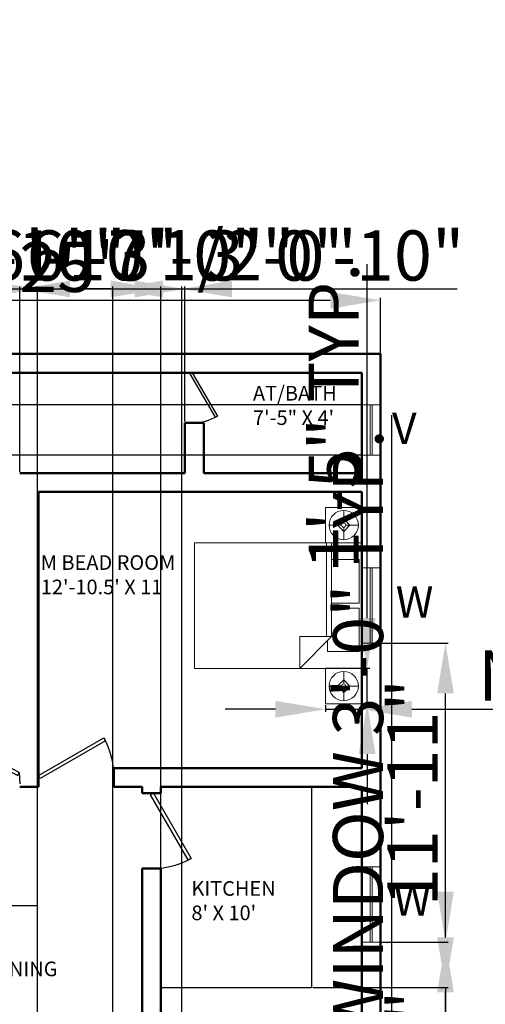
# Model space of a CAD drawing. Units: inches. Extents: x 1383 to 2465, y 1661 to 2415.
# Tile 3 of 4: x 1880 to 2102, y 1944 to 2415. Entities that reach past the tile are written whole.
import ezdxf

# ---------------------------------------------------------------- set-up
doc = ezdxf.new("R2010")
doc.units = ezdxf.units.IN
for name, color, linetype, lineweight in [('A-ANNO-DIMS', 2, 'Continuous', 18), ('A-ANNO-TEXT', 3, 'Continuous', 18), ('A-AREA-IDEN', 7, 'Continuous', 25), ('A-DOOR', 3, 'Continuous', 25), ('A-FLOR-FIXT', 9, 'Continuous', 25), ('A-FURN', 8, 'Continuous', 18), ('A-GLAZ', 4, 'Continuous', 18), ('A-WALL', 7, 'Continuous', 50)]:
    doc.layers.add(name, color=color, linetype=linetype, lineweight=lineweight)
doc.styles.get("Standard").update_dxf_attribs({"font": 'arial.ttf'})
doc.dimstyles.new('ISO-25', dxfattribs={"dimtxt": 24, "dimasz": 24, "dimexe": 1.25, "dimexo": 0.625, "dimtad": 1, "dimdec": 0, "dimlunit": 3, "dimtxsty": 'Standard', "dimcen": 2.5, "dimadec": 0, "dimazin": 0, "dimtfac": 1, "dimtdec": 0, "dimtmove": 0, "dimatfit": 3, "dimfxl": 1, "dimarcsym": 0})

# ---------------------------------------------------------------- blocks, each defined once
blk = doc.blocks.new('*U2')
for p, q in [((0, 0), (0, -6)), ((40, 0), (40, -6))]:
    blk.add_line(p, q)
blk.add_lwpolyline([(0, 0), (34.64, 20), (35.52, 18.48), (0.87, -1.52)], close=True)
blk.add_arc((0, 0), 40, 0, 30)
blk = doc.blocks.new('*U4')
for p, q in [((0, 0), (0, -6)), ((-40, 0), (-40, -6))]:
    blk.add_line(p, q)
blk.add_lwpolyline([(0, 0), (-34.64, 20), (-35.52, 18.48), (-0.88, -1.52)], close=True)
blk.add_arc((0, 0), 40, 150, 180)
blk = doc.blocks.new('*U5')
for p, q in [((-40, 0), (-40, 6)), ((0, 0), (0, 6))]:
    blk.add_line(p, q)
blk.add_lwpolyline([(0, 0), (-34.64, -20), (-35.52, -18.48), (-0.88, 1.52)], close=True)
blk.add_arc((0, 0), 40, 180, 210)
blk = doc.blocks.new('Bed - Queen')
for p, q in [((0, -80.00003), (0, 0)), ((0, 0), (59.99999, 0)), ((59.99999, 0), (59.99999, -80.00003)), ((7.99999, -1.2), (28.79998, -1.2)), ((7.99999, -14.4), (7.99999, -1.2)), ((28.79998, -1.2), (28.79998, -14.4)), ((31.19999, -1.2), (51.99999, -1.2)), ((31.19999, -14.4), (31.19999, -1.2)), ((51.99999, -1.2), (51.99999, -16.4)), ((0, -14.4), (44.8, -14.4)), ((44.8, -16.8), (0, -16.8)), ((59.99999, -29.6), (44.8, -14.4)), ((44.8, -14.4), (44.8, -29.6)), ((51.99999, -16.4), (46.79936, -16.4)), ((44.8, -29.6), (59.99999, -29.6)), ((59.99999, -80.00003), (0, -80.00003))]:
    blk.add_line(p, q)
blk = doc.blocks.new('*D12')
at = {"layer": 'A-ANNO-DIMS', "color": 0, "lineweight": -2, "transparency": 16777216}
for p, q in [((1752.19, 2255.79), (1752.19, 2282.04)), ((1776.19, 2280.79), (2028.19, 2280.79)), ((2052.19, 2255.79), (2052.19, 2282.04))]:
    blk.add_line(p, q, dxfattribs=at)
at = {"layer": 'A-ANNO-DIMS', "color": 0, "transparency": 16777216}
for points in [[(1776.19, 2284.79), (1776.19, 2276.79), (1752.19, 2280.79)], [(2028.19, 2284.79), (2028.19, 2276.79), (2052.19, 2280.79)]]:
    blk.add_solid(points, dxfattribs=at)
at = {"layer": 'Defpoints', "color": 0, "transparency": 16777216}
for p in [(2052.19, 2280.79), (1752.19, 2255.16), (2052.19, 2255.16)]:
    blk.add_point(p, dxfattribs=at)
at = {"layer": 'A-ANNO-DIMS', "color": 0, "transparency": 16777216, "insert": (1902.19, 2293.67), "char_height": 24, "attachment_point": 5}
blk.add_mtext("25'", dxfattribs=at)
blk = doc.blocks.new('WIN-36IN')
for p, q in [((0, 36), (9, 36)), ((0, 0), (0, 36)), ((4, 0), (4, 36)), ((5, 36), (5, 0)), ((9, 36), (9, 0)), ((9, 0), (0, 0))]:
    blk.add_line(p, q)
blk = doc.blocks.new('Lamp - Table')
for p, q in [((0, 7), (0, 1)), ((-1, 0), (-7, 0)), ((0, 3), (-3, 0)), ((-3, 0), (0, -3)), ((3, 0), (0, 3)), ((0, -3), (3, 0)), ((1, 0), (7, 0)), ((0, -1), (0, -7))]:
    blk.add_line(p, q)
for radius in [7, 1]:
    blk.add_circle((0, 0), radius)
blk = doc.blocks.new('NIGHTSTAND-WITH-LAMP')
blk.add_lwpolyline([(0, 0), (17.23, 0), (17.23, 16.98), (0, 16.98)], close=True)
blk.add_blockref('Lamp - Table', (8.62, 8.49))
blk = doc.blocks.new('*D16')
at = {"layer": 'A-ANNO-DIMS', "color": 0, "lineweight": -2, "transparency": 16777216}
for p, q in [((2025.96, 2087.24), (2025.96, 2084.03)), ((2043.19, 2087.24), (2043.19, 2084.03)), ((2001.96, 2085.28), (1977.96, 2085.28)), ((2025.96, 2085.28), (2043.19, 2085.28)), ((2067.19, 2085.28), (2464.82, 2085.28))]:
    blk.add_line(p, q, dxfattribs=at)
at = {"layer": 'A-ANNO-DIMS', "color": 0, "transparency": 16777216}
for points in [[(2001.96, 2089.28), (2001.96, 2081.28), (2025.96, 2085.28)], [(2067.19, 2089.28), (2067.19, 2081.28), (2043.19, 2085.28)]]:
    blk.add_solid(points, dxfattribs=at)
at = {"layer": 'Defpoints', "color": 0, "transparency": 16777216}
for p in [(2025.96, 2087.86), (2043.19, 2087.86), (2043.19, 2085.28)]:
    blk.add_point(p, dxfattribs=at)
at = {"layer": 'A-ANNO-DIMS', "color": 0, "transparency": 16777216, "insert": (2278.01, 2098.31), "char_height": 24, "attachment_point": 5}
blk.add_mtext('NIGHTSTAND 1\'-5" TYP.', dxfattribs=at)
blk = doc.blocks.new('*D17')
at = {"layer": 'A-ANNO-DIMS', "color": 0, "lineweight": -2, "transparency": 16777216}
for p, q in [((2045.78, 2128.84), (2045.78, 2298.12)), ((2043.82, 2104.84), (2047.03, 2104.84)), ((2045.78, 2087.86), (2045.78, 2104.84)), ((2043.82, 2087.86), (2047.03, 2087.86)), ((2045.78, 2063.86), (2045.78, 2039.86))]:
    blk.add_line(p, q, dxfattribs=at)
at = {"layer": 'A-ANNO-DIMS', "color": 0, "transparency": 16777216}
for points in [[(2041.78, 2128.84), (2049.78, 2128.84), (2045.78, 2104.84)], [(2041.78, 2063.86), (2049.78, 2063.86), (2045.78, 2087.86)]]:
    blk.add_solid(points, dxfattribs=at)
at = {"layer": 'Defpoints', "color": 0, "transparency": 16777216}
for p in [(2043.19, 2104.84), (2045.78, 2104.84), (2043.19, 2087.86)]:
    blk.add_point(p, dxfattribs=at)
at = {"layer": 'A-ANNO-DIMS', "color": 0, "transparency": 16777216, "insert": (2032.9, 2225.48), "char_height": 24, "attachment_point": 5, "rotation": 90}
blk.add_mtext('1\'-5" TYP.', dxfattribs=at)
blk = doc.blocks.new('*D18')
at = {"layer": 'A-ANNO-DIMS', "color": 0, "lineweight": -2, "transparency": 16777216}
for p, q in [((2057.59, 1896.91), (2057.59, 2225.86)), ((2052.82, 1872.91), (2058.84, 1872.91)), ((2057.59, 1836.91), (2057.59, 1872.91)), ((2052.82, 1836.91), (2058.84, 1836.91)), ((2057.59, 1812.91), (2057.59, 1788.91))]:
    blk.add_line(p, q, dxfattribs=at)
at = {"layer": 'A-ANNO-DIMS', "color": 0, "transparency": 16777216}
for points in [[(2053.59, 1896.91), (2061.59, 1896.91), (2057.59, 1872.91)], [(2053.59, 1812.91), (2061.59, 1812.91), (2057.59, 1836.91)]]:
    blk.add_solid(points, dxfattribs=at)
at = {"layer": 'Defpoints', "color": 0, "transparency": 16777216}
for p in [(2052.19, 1872.91), (2057.59, 1872.91), (2052.19, 1836.91)]:
    blk.add_point(p, dxfattribs=at)
at = {"layer": 'A-ANNO-DIMS', "color": 0, "transparency": 16777216, "insert": (2044.54, 2073.39), "char_height": 24, "attachment_point": 5, "rotation": 90}
blk.add_mtext('WINDOW 3\'-0" TYP.', dxfattribs=at)
blk = doc.blocks.new('*D32')
at = {"layer": 'A-ANNO-DIMS', "color": 0, "lineweight": -2, "transparency": 16777216}
for p, q in [((2052.82, 1973.98), (2084.49, 1973.98)), ((2083.24, 1860.91), (2083.24, 1949.98)), ((2052.82, 1836.91), (2084.49, 1836.91))]:
    blk.add_line(p, q, dxfattribs=at)
at = {"layer": 'A-ANNO-DIMS', "color": 0, "transparency": 16777216}
for points in [[(2079.24, 1949.98), (2087.24, 1949.98), (2083.24, 1973.98)], [(2079.24, 1860.91), (2087.24, 1860.91), (2083.24, 1836.91)]]:
    blk.add_solid(points, dxfattribs=at)
at = {"layer": 'Defpoints', "color": 0, "transparency": 16777216}
for p in [(2052.19, 1973.98), (2083.24, 1973.98), (2052.19, 1836.91)]:
    blk.add_point(p, dxfattribs=at)
at = {"layer": 'A-ANNO-DIMS', "color": 0, "transparency": 16777216, "insert": (2070.36, 1905.44), "char_height": 24, "attachment_point": 5, "rotation": 90}
blk.add_mtext('11\'-5"', dxfattribs=at)
blk = doc.blocks.new('*D33')
at = {"layer": 'A-ANNO-DIMS', "color": 0, "lineweight": -2, "transparency": 16777216}
for p, q in [((2052.82, 2116.87), (2084.49, 2116.87)), ((2083.24, 1997.98), (2083.24, 2092.87)), ((2052.82, 1973.98), (2084.49, 1973.98))]:
    blk.add_line(p, q, dxfattribs=at)
at = {"layer": 'A-ANNO-DIMS', "color": 0, "transparency": 16777216}
for points in [[(2079.24, 2092.87), (2087.24, 2092.87), (2083.24, 2116.87)], [(2079.24, 1997.98), (2087.24, 1997.98), (2083.24, 1973.98)]]:
    blk.add_solid(points, dxfattribs=at)
at = {"layer": 'Defpoints', "color": 0, "transparency": 16777216}
for p in [(2052.19, 2116.87), (2083.24, 2116.87), (2052.19, 1973.98)]:
    blk.add_point(p, dxfattribs=at)
at = {"layer": 'A-ANNO-DIMS', "color": 0, "transparency": 16777216, "insert": (2070.57, 2045.42), "char_height": 24, "attachment_point": 5, "rotation": 90}
blk.add_mtext('11\'-11"', dxfattribs=at)
blk = doc.blocks.new('*D34')
at = {"layer": 'A-ANNO-DIMS', "color": 0, "lineweight": -2, "transparency": 16777216}
for p, q in [((1721.14, 2254.82), (1721.14, 2344.28)), ((2042.57, 2230.82), (1719.89, 2230.82)), ((1721.14, 2206.82), (1721.14, 2230.82)), ((2042.57, 2206.82), (1719.89, 2206.82)), ((1721.14, 2182.82), (1721.14, 2158.82))]:
    blk.add_line(p, q, dxfattribs=at)
at = {"layer": 'A-ANNO-DIMS', "color": 0, "transparency": 16777216}
for points in [[(1717.14, 2254.82), (1725.14, 2254.82), (1721.14, 2230.82)], [(1717.14, 2182.82), (1725.14, 2182.82), (1721.14, 2206.82)]]:
    blk.add_solid(points, dxfattribs=at)
at = {"layer": 'Defpoints', "color": 0, "transparency": 16777216}
for p in [(1721.14, 2230.82), (2043.19, 2230.82), (2043.19, 2206.82)]:
    blk.add_point(p, dxfattribs=at)
at = {"layer": 'A-ANNO-DIMS', "color": 0, "transparency": 16777216, "insert": (1708.26, 2311.55), "char_height": 24, "attachment_point": 5, "rotation": 90}
blk.add_mtext('2\'-0"', dxfattribs=at)
blk = doc.blocks.new('*D35')
at = {"layer": 'A-ANNO-DIMS', "color": 0, "lineweight": -2, "transparency": 16777216}
for p, q in [((1721.14, 2270.16), (1721.14, 2412.87)), ((2042.57, 2246.16), (1719.89, 2246.16)), ((1721.14, 2230.82), (1721.14, 2246.16)), ((2042.57, 2230.82), (1719.89, 2230.82)), ((1721.14, 2206.82), (1721.14, 2182.82))]:
    blk.add_line(p, q, dxfattribs=at)
at = {"layer": 'A-ANNO-DIMS', "color": 0, "transparency": 16777216}
for points in [[(1717.14, 2270.16), (1725.14, 2270.16), (1721.14, 2246.16)], [(1717.14, 2206.82), (1725.14, 2206.82), (1721.14, 2230.82)]]:
    blk.add_solid(points, dxfattribs=at)
at = {"layer": 'Defpoints', "color": 0, "transparency": 16777216}
for p in [(1721.14, 2246.16), (2043.19, 2246.16), (2043.19, 2230.82)]:
    blk.add_point(p, dxfattribs=at)
at = {"layer": 'A-ANNO-DIMS', "color": 0, "transparency": 16777216, "insert": (1708.1, 2353.52), "char_height": 24, "attachment_point": 5, "rotation": 90}
blk.add_mtext('1\'-3 1/2"', dxfattribs=at)
blk = doc.blocks.new('*D38')
at = {"layer": 'A-ANNO-DIMS', "color": 0, "lineweight": -2, "transparency": 16777216}
for p, q in [((1761.19, 2198.79), (1761.19, 2287.46)), ((1785.19, 2286.21), (1819.69, 2286.21)), ((1843.69, 2198.79), (1843.69, 2287.46)), ((1843.69, 2286.21), (2007.44, 2286.21))]:
    blk.add_line(p, q, dxfattribs=at)
at = {"layer": 'A-ANNO-DIMS', "color": 0, "transparency": 16777216}
for points in [[(1785.19, 2290.21), (1785.19, 2282.21), (1761.19, 2286.21)], [(1819.69, 2290.21), (1819.69, 2282.21), (1843.69, 2286.21)]]:
    blk.add_solid(points, dxfattribs=at)
at = {"layer": 'Defpoints', "color": 0, "transparency": 16777216}
for p in [(1843.69, 2286.21), (1761.19, 2198.16), (1843.69, 2198.16)]:
    blk.add_point(p, dxfattribs=at)
at = {"layer": 'A-ANNO-DIMS', "color": 0, "transparency": 16777216, "insert": (1937.57, 2299.25), "char_height": 24, "attachment_point": 5}
blk.add_mtext('6\'-10 1/2"', dxfattribs=at)
blk = doc.blocks.new('*D39')
at = {"layer": 'A-ANNO-DIMS', "color": 0, "lineweight": -2, "transparency": 16777216}
for p, q in [((1819.69, 2286.21), (1795.69, 2286.21)), ((1843.69, 2198.79), (1843.69, 2287.46)), ((1843.69, 2286.21), (1879.69, 2286.21)), ((1879.69, 2198.79), (1879.69, 2287.46)), ((1903.69, 2286.21), (1992.73, 2286.21))]:
    blk.add_line(p, q, dxfattribs=at)
at = {"layer": 'A-ANNO-DIMS', "color": 0, "transparency": 16777216}
for points in [[(1819.69, 2290.21), (1819.69, 2282.21), (1843.69, 2286.21)], [(1903.69, 2290.21), (1903.69, 2282.21), (1879.69, 2286.21)]]:
    blk.add_solid(points, dxfattribs=at)
at = {"layer": 'Defpoints', "color": 0, "transparency": 16777216}
for p in [(1879.69, 2286.21), (1843.69, 2198.16), (1879.69, 2198.16)]:
    blk.add_point(p, dxfattribs=at)
at = {"layer": 'A-ANNO-DIMS', "color": 0, "transparency": 16777216, "insert": (1960.21, 2299.1), "char_height": 24, "attachment_point": 5}
blk.add_mtext('3\'-0"', dxfattribs=at)
blk = doc.blocks.new('*D40')
at = {"layer": 'A-ANNO-DIMS', "color": 0, "lineweight": -2, "transparency": 16777216}
for p, q in [((1879.69, 2198.79), (1879.69, 2287.46)), ((1903.69, 2286.21), (1934.69, 2286.21)), ((1958.69, 2222.79), (1958.69, 2287.46))]:
    blk.add_line(p, q, dxfattribs=at)
at = {"layer": 'A-ANNO-DIMS', "color": 0, "transparency": 16777216}
for points in [[(1903.69, 2290.21), (1903.69, 2282.21), (1879.69, 2286.21)], [(1934.69, 2290.21), (1934.69, 2282.21), (1958.69, 2286.21)]]:
    blk.add_solid(points, dxfattribs=at)
at = {"layer": 'Defpoints', "color": 0, "transparency": 16777216}
for p in [(1958.69, 2286.21), (1958.69, 2222.16), (1879.69, 2198.16)]:
    blk.add_point(p, dxfattribs=at)
at = {"layer": 'A-ANNO-DIMS', "color": 0, "transparency": 16777216, "insert": (1919.19, 2299.09), "char_height": 24, "attachment_point": 5}
blk.add_mtext('6\'-7"', dxfattribs=at)
blk = doc.blocks.new('*D43')
at = {"layer": 'A-ANNO-DIMS', "color": 0, "lineweight": -2, "transparency": 16777216}
for p, q in [((1923.19, 2286.21), (1899.19, 2286.21)), ((1947.19, 1919.79), (1947.19, 2287.46)), ((1947.19, 2286.21), (1957.19, 2286.21)), ((1957.19, 1919.79), (1957.19, 2287.46)), ((1981.19, 2286.21), (2088.89, 2286.21))]:
    blk.add_line(p, q, dxfattribs=at)
at = {"layer": 'A-ANNO-DIMS', "color": 0, "transparency": 16777216}
for points in [[(1923.19, 2290.21), (1923.19, 2282.21), (1947.19, 2286.21)], [(1981.19, 2290.21), (1981.19, 2282.21), (1957.19, 2286.21)]]:
    blk.add_solid(points, dxfattribs=at)
at = {"layer": 'Defpoints', "color": 0, "transparency": 16777216}
for p in [(1957.19, 2286.21), (1947.19, 1919.16), (1957.19, 1919.16)]:
    blk.add_point(p, dxfattribs=at)
at = {"layer": 'A-ANNO-DIMS', "color": 0, "transparency": 16777216, "insert": (2047.04, 2299.09), "char_height": 24, "attachment_point": 5}
blk.add_mtext('0\'-10"', dxfattribs=at)
blk = doc.blocks.new('*D47')
at = {"layer": 'A-ANNO-DIMS', "color": 0, "lineweight": -2, "transparency": 16777216}
for p, q in [((1721.14, 1883.16), (1721.14, 1972.21)), ((1946.57, 1883.16), (1719.89, 1883.16)), ((1721.14, 1847.16), (1721.14, 1859.16)), ((1946.57, 1823.16), (1719.89, 1823.16))]:
    blk.add_line(p, q, dxfattribs=at)
at = {"layer": 'A-ANNO-DIMS', "color": 0, "transparency": 16777216}
for points in [[(1717.14, 1859.16), (1725.14, 1859.16), (1721.14, 1883.16)], [(1717.14, 1847.16), (1725.14, 1847.16), (1721.14, 1823.16)]]:
    blk.add_solid(points, dxfattribs=at)
at = {"layer": 'Defpoints', "color": 0, "transparency": 16777216}
for p in [(1721.14, 1883.16), (1947.19, 1883.16), (1947.19, 1823.16)]:
    blk.add_point(p, dxfattribs=at)
at = {"layer": 'A-ANNO-DIMS', "color": 0, "transparency": 16777216, "insert": (1708.26, 1939.69), "char_height": 24, "attachment_point": 5, "rotation": 90}
blk.add_mtext('5\'-0"', dxfattribs=at)
blk = doc.blocks.new('*D49')
at = {"layer": 'A-ANNO-DIMS', "color": 0, "lineweight": -2, "transparency": 16777216}
for p, q in [((1737.19, 2286.21), (1713.19, 2286.21)), ((1761.19, 1991.92), (1761.19, 2287.46)), ((1761.19, 2286.21), (1795.19, 2286.21)), ((1795.19, 2033.92), (1795.19, 2287.46)), ((1819.19, 2286.21), (1927.3, 2286.21))]:
    blk.add_line(p, q, dxfattribs=at)
at = {"layer": 'A-ANNO-DIMS', "color": 0, "transparency": 16777216}
for points in [[(1737.19, 2290.21), (1737.19, 2282.21), (1761.19, 2286.21)], [(1819.19, 2290.21), (1819.19, 2282.21), (1795.19, 2286.21)]]:
    blk.add_solid(points, dxfattribs=at)
at = {"layer": 'Defpoints', "color": 0, "transparency": 16777216}
for p in [(1795.19, 2286.21), (1795.19, 2033.3), (1761.19, 1991.3)]:
    blk.add_point(p, dxfattribs=at)
at = {"layer": 'A-ANNO-DIMS', "color": 0, "transparency": 16777216, "insert": (1885.25, 2299.09), "char_height": 24, "attachment_point": 5}
blk.add_mtext('2\'-10"', dxfattribs=at)
blk = doc.blocks.new('*D50')
at = {"layer": 'A-ANNO-DIMS', "color": 0, "lineweight": -2, "transparency": 16777216}
for p, q in [((1864.19, 2286.21), (1840.19, 2286.21)), ((1888.19, 1919.79), (1888.19, 2287.46)), ((1888.19, 2286.21), (1924.19, 2286.21)), ((1924.19, 1919.79), (1924.19, 2287.46)), ((1948.19, 2286.21), (2037.23, 2286.21))]:
    blk.add_line(p, q, dxfattribs=at)
at = {"layer": 'A-ANNO-DIMS', "color": 0, "transparency": 16777216}
for points in [[(1864.19, 2290.21), (1864.19, 2282.21), (1888.19, 2286.21)], [(1948.19, 2290.21), (1948.19, 2282.21), (1924.19, 2286.21)]]:
    blk.add_solid(points, dxfattribs=at)
at = {"layer": 'Defpoints', "color": 0, "transparency": 16777216}
for p in [(1924.19, 2286.21), (1888.19, 1919.16), (1924.19, 1919.16)]:
    blk.add_point(p, dxfattribs=at)
at = {"layer": 'A-ANNO-DIMS', "color": 0, "transparency": 16777216, "insert": (2004.71, 2299.1), "char_height": 24, "attachment_point": 5}
blk.add_mtext('3\'-0"', dxfattribs=at)
blk = doc.blocks.new('*D52')
at = {"layer": 'A-ANNO-DIMS', "color": 0, "lineweight": -2, "transparency": 16777216}
for p, q in [((2083.24, 1976.16), (2083.24, 2000.16)), ((2019.82, 1952.16), (2084.49, 1952.16)), ((2083.24, 1952.16), (2083.24, 1928.16)), ((2043.82, 1928.16), (2084.49, 1928.16)), ((2083.24, 1904.16), (2083.24, 1814.7))]:
    blk.add_line(p, q, dxfattribs=at)
at = {"layer": 'A-ANNO-DIMS', "color": 0, "transparency": 16777216}
for points in [[(2079.24, 1976.16), (2087.24, 1976.16), (2083.24, 1952.16)], [(2079.24, 1904.16), (2087.24, 1904.16), (2083.24, 1928.16)]]:
    blk.add_solid(points, dxfattribs=at)
at = {"layer": 'Defpoints', "color": 0, "transparency": 16777216}
for p in [(2019.19, 1952.16), (2043.19, 1928.16), (2083.24, 1928.16)]:
    blk.add_point(p, dxfattribs=at)
at = {"layer": 'A-ANNO-DIMS', "color": 0, "transparency": 16777216, "insert": (2070.36, 1847.43), "char_height": 24, "attachment_point": 5, "rotation": 90}
blk.add_mtext('2\'-0"', dxfattribs=at)
blk = doc.blocks.new('*D53')
at = {"layer": 'A-ANNO-DIMS', "color": 0, "lineweight": -2, "transparency": 16777216}
for p, q in [((1721.14, 1886.16), (1721.14, 1975.19)), ((1887.57, 1862.16), (1719.89, 1862.16)), ((1721.14, 1826.16), (1721.14, 1862.16)), ((1887.57, 1826.16), (1719.89, 1826.16)), ((1721.14, 1802.16), (1721.14, 1778.16))]:
    blk.add_line(p, q, dxfattribs=at)
at = {"layer": 'A-ANNO-DIMS', "color": 0, "transparency": 16777216}
for points in [[(1717.14, 1886.16), (1725.14, 1886.16), (1721.14, 1862.16)], [(1717.14, 1802.16), (1725.14, 1802.16), (1721.14, 1826.16)]]:
    blk.add_solid(points, dxfattribs=at)
at = {"layer": 'Defpoints', "color": 0, "transparency": 16777216}
for p in [(1721.14, 1862.16), (1888.19, 1862.16), (1888.19, 1826.16)]:
    blk.add_point(p, dxfattribs=at)
at = {"layer": 'A-ANNO-DIMS', "color": 0, "transparency": 16777216, "insert": (1708.26, 1942.68), "char_height": 24, "attachment_point": 5, "rotation": 90}
blk.add_mtext('3\'-0"', dxfattribs=at)
blk = doc.blocks.new('*D54')
at = {"layer": 'A-ANNO-DIMS', "color": 0, "lineweight": -2, "transparency": 16777216}
for p, q in [((1612.53, 1991.3), (1743.19, 1991.3)), ((1888.39, 1991.3), (1767.19, 1991.3))]:
    blk.add_line(p, q, dxfattribs=at)
at = {"layer": 'A-ANNO-DIMS', "color": 0, "transparency": 16777216}
blk.add_solid([(1743.19, 1995.3), (1743.19, 1987.3), (1767.19, 1991.3)], dxfattribs=at)
at = {"layer": 'Defpoints', "color": 0, "transparency": 16777216}
for p in [(1767.19, 1991.3), (1888.39, 1991.3)]:
    blk.add_point(p, dxfattribs=at)
at = {"layer": 'A-ANNO-DIMS', "color": 0, "transparency": 16777216, "insert": (1665.86, 2004.17), "char_height": 24, "attachment_point": 5, "rotation": 359.9999}
blk.add_mtext('R10\'-1"', dxfattribs=at)

msp = doc.modelspace()

# ---------------------------------------------------------------- linework, layer by layer
at = {"layer": 'A-FLOR-FIXT'}
for p in [(2019.19, 2048.16), (1947.19, 1952.16)]:
    msp.add_line(p, (2019.19, 1952.16), dxfattribs=at)
at = {"layer": 'A-GLAZ'}
for p, q in [((2043.19, 2230.82), (2052.19, 2230.82)), ((2043.19, 2206.82), (2043.19, 2230.82)), ((2047.19, 2206.82), (2047.19, 2230.82)), ((2048.19, 2230.82), (2048.19, 2206.82)), ((2052.19, 2230.82), (2052.19, 2206.82)), ((2052.19, 2206.82), (2043.19, 2206.82))]:
    msp.add_line(p, q, dxfattribs=at)
at = {"layer": 'A-WALL'}
for p, q in [((1761.19, 2246.16), (2043.19, 2246.16)), ((1958.69, 2246.16), (1967.69, 2246.16)), ((2043.19, 2246.16), (2043.19, 2198.16)), ((1958.69, 2198.16), (1958.69, 2222.16)), ((1958.69, 2222.16), (1967.69, 2222.16)), ((1967.69, 2198.16), (1967.69, 2222.16)), ((1879.69, 2198.16), (1958.69, 2198.16)), ((1967.69, 2198.16), (2043.19, 2198.16)), ((1888.69, 2189.16), (1888.69, 2048.16)), ((1888.69, 2189.16), (2043.19, 2189.16)), ((2043.19, 2189.16), (2043.19, 2057.16)), ((1888.69, 2048.16), (1888.69, 2057.16)), ((1924.69, 2048.16), (1924.69, 2057.16)), ((1924.69, 2057.16), (2043.19, 2057.16)), ((1879.69, 2048.16), (1888.69, 2048.16)), ((1924.69, 2048.16), (1938.19, 2048.16)), ((1938.19, 2048.16), (1938.19, 2045.16)), ((1947.19, 2048.16), (1947.19, 2045.16)), ((1947.19, 2048.16), (2043.19, 2048.16)), ((2043.19, 2048.16), (2043.19, 1928.16)), ((1938.19, 2045.16), (1947.19, 2045.16)), ((1938.19, 2009.16), (1947.19, 2009.16)), ((1938.19, 2009.16), (1938.19, 1928.16)), ((1947.19, 2009.16), (1947.19, 1928.16))]:
    msp.add_line(p, q, dxfattribs=at)
msp.add_lwpolyline([(1752.19, 2255.16), (2052.19, 2255.16), (2052.19, 1715.16), (1752.19, 1715.16)], close=True, dxfattribs=at)

# ---------------------------------------------------------------- block references
at = {"layer": 'A-DOOR'}
for name, p, xscale, yscale, zscale, rotation in [('*U2', (1962.17, 2246.16), 0.5995524082297461, 0.5995524082297461, 0.5995524082297461, 270.2900542956196), ('*U4', (1879.48, 2054.97), 0.9006830181943749, 0.9006830181943749, 0.9006830181943749, 2.231491455052545), ('*U5', (1888.69, 2053.56), 0.9, 0.9, 0.9, 180), ('*U2', (1943.59, 2045.16), 0.9, 0.9, 0.9, 270)]:
    msp.add_blockref(name, p, dxfattribs=dict(at, xscale=xscale, yscale=yscale, zscale=zscale, rotation=rotation))
at = {"layer": 'A-FURN'}
for p in [(2025.96, 2164.81), (2025.96, 2087.86)]:
    msp.add_blockref('NIGHTSTAND-WITH-LAMP', p, dxfattribs=at)
at = {"layer": 'A-FURN', "rotation": 270}
msp.add_blockref('Bed - Queen', (2043.19, 2164.81), dxfattribs=at)
at = {"layer": 'A-GLAZ'}
for p in [(2043.19, 2116.87), (2043.19, 1973.98)]:
    msp.add_blockref('WIN-36IN', p, dxfattribs=at)

# ---------------------------------------------------------------- texts
at = {"layer": 'A-ANNO-TEXT', "char_height": 15, "attachment_point": 1}
for s, insert in [('{\\fArial|b1|i0|c0|p34;V}', (2057.67, 2227.07)), ('{\\fArial|b1|i0|c0|p34;W}', (2059.49, 2144.02)), ('{\\fArial|b1|i0|c0|p34;W}', (2058.41, 2001.57))]:
    msp.add_mtext_dynamic_manual_height_columns(s, width=53.5912, gutter_width=12.5, heights=[38.86], dxfattribs=dict(at, insert=insert))
at = {"layer": 'A-AREA-IDEN', "char_height": 7, "attachment_point": 1}
for s, width, heights, insert in [('{\\fArial|b1|i0|c0|p34;AT/BATH\\P7\'-5" X 4\'}', 53.5912, [38.86], (1991.21, 2239.86)), ("{\\fArial|b1|i0|c0|p34;M BEAD ROOM\\P12'-10.5' X 11}", 82.2642, [71.06], (1889.77, 2158.91)), ("{\\fArial|b1|i0|c0|p34;KITCHEN\\P8' X 10'}", 53.5912, [38.86], (1961.79, 2003.08)), ('{\\fArial|b1|i0|c0|p34;DRAWING /DINING\\P15\'10.5" X 10\'}', 95.0663, [44.26], (1816.2, 1964.61))]:
    msp.add_mtext_dynamic_manual_height_columns(s, width=width, gutter_width=12.5, heights=heights, dxfattribs=dict(at, insert=insert))

# ---------------------------------------------------------------- dimensions: what is measured, and where the dimension line sits
at = {"layer": 'A-ANNO-DIMS'}
for base, p1, p2, picture, middle in [((1721.14, 2246.16), (2043.19, 2230.82), (2043.19, 2246.16), '*D35', (1708.1, 2353.52)), ((1721.14, 2230.82), (2043.19, 2206.82), (2043.19, 2230.82), '*D34', (1708.26, 2311.55)), ((2083.24, 2116.87), (2052.19, 1973.98), (2052.19, 2116.87), '*D33', (2070.57, 2045.42)), ((2083.24, 1928.16), (2019.19, 1952.16), (2043.19, 1928.16), '*D52', (2070.36, 1847.43)), ((1721.14, 1862.16), (1888.19, 1826.16), (1888.19, 1862.16), '*D53', (1708.26, 1942.68)), ((1721.14, 1883.16), (1947.19, 1823.16), (1947.19, 1883.16), '*D47', (1708.26, 1939.69)), ((2083.24, 1973.98), (2052.19, 1836.91), (2052.19, 1973.98), '*D32', (2070.36, 1905.44))]:
    dim = msp.add_linear_dim(base=base, p1=p1, p2=p2, angle=90, dimstyle='ISO-25', override={"dimdec": 1, "dimlfac": 1, "dimrnd": 0, "dimzin": 1, "dimdsep": 46, "dimlunit": 4, "dimfrac": 2}, dxfattribs=at)
    dim.commit()
    dim.dimension.update_dxf_attribs({"geometry": picture, "text_midpoint": middle})
for base, p1, p2, override, picture, middle in [((1843.69, 2286.21), (1761.19, 2198.16), (1843.69, 2198.16), {"dimdec": 1, "dimlfac": 1, "dimrnd": 0, "dimzin": 1, "dimdsep": 46, "dimlunit": 4, "dimfrac": 2}, '*D38', (1937.57, 2299.25)), ((1795.19, 2286.21), (1761.19, 1991.3), (1795.19, 2033.3), {"dimdec": 1, "dimlfac": 1, "dimrnd": 0, "dimzin": 1, "dimdsep": 46, "dimlunit": 4, "dimfrac": 2}, '*D49', (1885.25, 2299.09)), ((1879.69, 2286.21), (1843.69, 2198.16), (1879.69, 2198.16), {"dimdec": 1, "dimlfac": 1, "dimrnd": 0, "dimzin": 1, "dimdsep": 46, "dimlunit": 4, "dimfrac": 2}, '*D39', (1960.21, 2299.1)), ((1924.19, 2286.21), (1888.19, 1919.16), (1924.19, 1919.16), {"dimdec": 1, "dimlfac": 1, "dimrnd": 0, "dimzin": 1, "dimdsep": 46, "dimlunit": 4, "dimfrac": 2}, '*D50', (2004.71, 2299.1)), ((1958.69, 2286.21), (1879.69, 2198.16), (1958.69, 2222.16), {"dimdec": 1, "dimlfac": 1, "dimrnd": 0, "dimzin": 1, "dimdsep": 46, "dimlunit": 4, "dimfrac": 2}, '*D40', (1919.19, 2299.09)), ((1957.19, 2286.21), (1947.19, 1919.16), (1957.19, 1919.16), {"dimdec": 1, "dimlfac": 1, "dimrnd": 0, "dimzin": 1, "dimdsep": 46, "dimlunit": 4, "dimfrac": 2}, '*D43', (2047.04, 2299.09)), ((2052.19, 2280.79), (1752.19, 2255.16), (2052.19, 2255.16), {"dimclrd": 0, "dimclre": 0, "dimclrt": 0}, '*D12', (1902.19, 2293.67))]:
    dim = msp.add_linear_dim(base=base, p1=p1, p2=p2, dimstyle='ISO-25', override=override, dxfattribs=at)
    dim.commit()
    dim.dimension.update_dxf_attribs({"geometry": picture, "text_midpoint": middle})
for base, p1, p2, text, picture, middle in [((2045.78, 2104.84), (2043.19, 2087.86), (2043.19, 2104.84), '<> TYP.', '*D17', (2032.9, 2225.48)), ((2057.59, 1872.91), (2052.19, 1836.91), (2052.19, 1872.91), 'WINDOW <> TYP.', '*D18', (2044.54, 2073.39))]:
    dim = msp.add_linear_dim(base=base, p1=p1, p2=p2, angle=90, text=text, dimstyle='ISO-25', override={"dimdec": 1, "dimlfac": 1, "dimrnd": 0, "dimzin": 1, "dimdsep": 46, "dimlunit": 4, "dimfrac": 2}, dxfattribs=at)
    dim.commit()
    dim.dimension.update_dxf_attribs({"geometry": picture, "text_midpoint": middle})
dim = msp.add_linear_dim(base=(2043.19, 2085.28), p1=(2025.96, 2087.86), p2=(2043.19, 2087.86), text='NIGHTSTAND <> TYP.', dimstyle='ISO-25', override={"dimdec": 1, "dimlfac": 1, "dimrnd": 0, "dimzin": 1, "dimdsep": 46, "dimlunit": 4, "dimfrac": 2}, dxfattribs=at)
dim.commit()
dim.dimension.update_dxf_attribs({"geometry": '*D16', "text_midpoint": (2278.01, 2098.31)})
dim = msp.add_radius_dim(center=(1888.39, 1991.3), mpoint=(1767.19, 1991.3), dimstyle='ISO-25', override={"dimdec": 1, "dimlfac": 1, "dimrnd": 0, "dimzin": 1, "dimdsep": 46, "dimlunit": 4, "dimfrac": 2}, dxfattribs=at)
dim.commit()
dim.dimension.update_dxf_attribs({"geometry": '*D54', "text_midpoint": (1665.86, 2004.17)})

doc.saveas('drawing.dxf')
